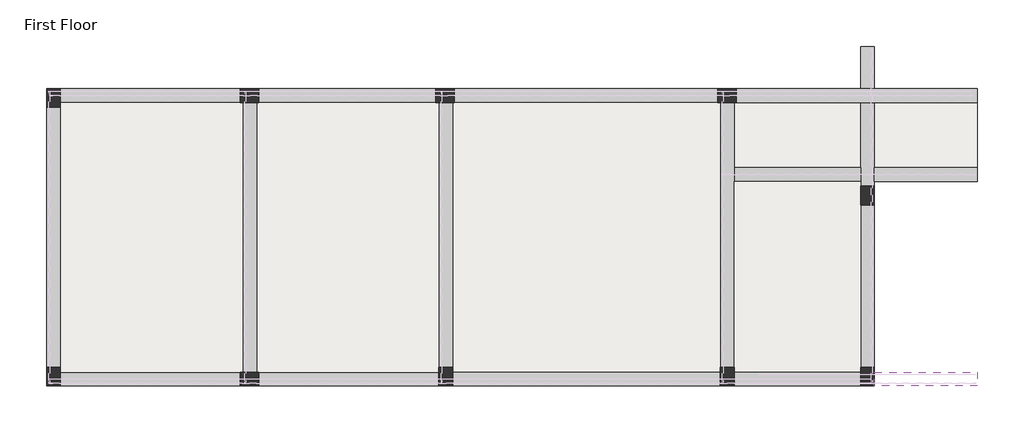
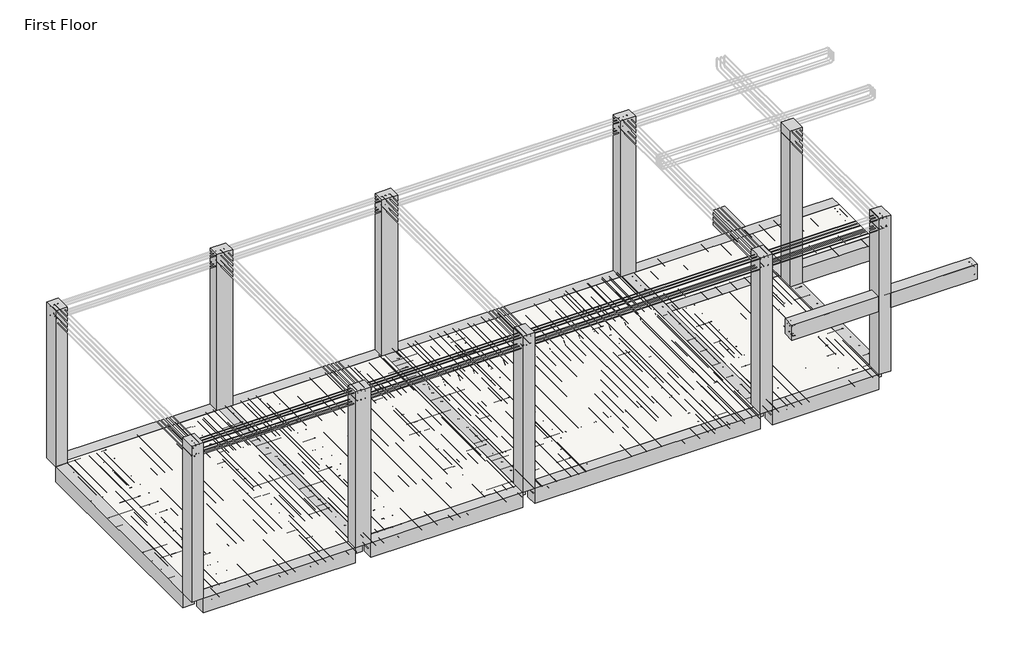
# One storey, part 1 of 4: 10 columns, 9 beams, 5 slabs.
"""IFC4 building model written with IfcOpenShell, lengths in millimetres."""

from ifc_helpers import new_model, si_unit, frame, origin, place, context, project, spatial, polyline, outline, extrude, faceted_brep, element, save

model = new_model("IFC4")

# Units and contexts
model_context = context("Model", 3, world=origin())
ifc_project = project(units=[si_unit("LENGTHUNIT", "METRE", prefix="MILLI")], contexts=[model_context])

# Site, building, storey
site = spatial("IfcSite", under=ifc_project)
building = spatial("IfcBuilding", under=site)
storey = spatial("IfcBuildingStorey", under=building, Name="First Floor", Elevation=3200.4)

# Beams
placement = place(None, origin())
element("IfcBeam", 1, ObjectType="M_Concrete-Rectangular Beam : 9\" X12\"", at=placement, inside=storey, context=model_context, shape_type="Brep", body=[
    faceted_brep([(3956.0882476, 186.4334631, 3200.4), (3956.0882476, 415.0334631, 3200.4), (1885.9882476, 415.0334631, 3200.4), (1885.9882476, 186.4334631, 3200.4), (3956.0882476, 186.4334631, 2895.6), (1885.9882476, 186.4334631, 2895.6), (3956.0882476, 415.0334631, 2895.6), (1885.9882476, 415.0334631, 2895.6), (3956.0882476, 415.0334631, 3048.0), (1885.9882476, 415.0334631, 3048.0)], [[[0, 1, 2, 3]], [[4, 0, 3, 5]], [[6, 4, 5, 7]], [[1, 8, 6, 7, 9, 2]], [[1, 0, 4, 6, 8]], [[3, 2, 9, 7, 5]]]),
    faceted_brep([(-9150.3117524, 186.4334631, 3200.4), (-9150.3117524, 415.0334631, 3200.4), (-9150.3117524, 415.0334631, 3048.0), (-9150.3117524, 415.0334631, 2895.6), (-9150.3117524, 186.4334631, 2895.6), (-6203.9117524, 415.0334631, 3200.4), (-6203.9117524, 186.4334631, 3200.4), (-6203.9117524, 186.4334631, 2895.6), (-6203.9117524, 415.0334631, 2895.6)], [[[0, 1, 2, 3, 4]], [[5, 6, 7, 8]], [[1, 0, 6, 5]], [[0, 4, 7, 6]], [[4, 3, 8, 7]], [[3, 2, 1, 5, 8]]]),
    faceted_brep([(-5899.1117524, 186.4334631, 3200.4), (-5899.1117524, 415.0334631, 3200.4), (-5899.1117524, 415.0334631, 2895.6), (-5899.1117524, 186.4334631, 2895.6), (-2952.7117524, 415.0334631, 3200.4), (-2952.7117524, 186.4334631, 3200.4), (-2952.7117524, 186.4334631, 2895.6), (-2952.7117524, 415.0334631, 2895.6), (-2952.7117524, 415.0334631, 3048.0)], [[[0, 1, 2, 3]], [[4, 5, 6, 7, 8]], [[1, 0, 5, 4]], [[0, 3, 6, 5]], [[3, 2, 7, 6]], [[2, 1, 4, 8, 7]]]),
    faceted_brep([(-2724.1117524, 186.4334631, 3200.4), (-2724.1117524, 415.0334631, 3200.4), (-2724.1117524, 415.0334631, 3048.0), (-2724.1117524, 415.0334631, 2895.6), (-2724.1117524, 186.4334631, 2895.6), (1657.3882476, 415.0334631, 3200.4), (1657.3882476, 186.4334631, 3200.4), (1657.3882476, 186.4334631, 2895.6), (1657.3882476, 415.0334631, 2895.6), (1657.3882476, 415.0334631, 3048.0)], [[[0, 1, 2, 3, 4]], [[5, 6, 7, 8, 9]], [[1, 0, 6, 5]], [[0, 4, 7, 6]], [[4, 3, 8, 7]], [[3, 2, 1, 5, 9, 8]]]),
])
element("IfcBeam", 2, ObjectType="M_Concrete-Rectangular Beam : 9\" X12\"", at=placement, inside=storey, context=model_context, shape_type="Brep", body=[
    faceted_brep([(3956.0882476, 5755.2386934, 3200.4), (4184.6882476, 5755.2386934, 3200.4), (4184.6882476, 5755.2386934, 2895.6), (3956.0882476, 5755.2386934, 2895.6), (3956.0882476, 5063.2334631, 3200.4), (4184.6882476, 5063.2334631, 3200.4), (4184.6882476, 5063.2334631, 2895.6), (3956.0882476, 5063.2334631, 2895.6)], [[[0, 1, 2, 3]], [[1, 0, 4, 5]], [[2, 1, 5, 6]], [[3, 2, 6, 7]], [[0, 3, 7, 4]], [[5, 4, 7, 6]]]),
    faceted_brep([(4184.6882476, 491.2334631, 3200.4), (3956.0882476, 491.2334631, 3200.4), (3956.0882476, 491.2334631, 2895.6), (4184.6882476, 491.2334631, 2895.6), (3956.0882476, 3158.2334631, 3200.4), (4184.6882476, 3158.2334631, 3200.4), (4184.6882476, 3158.2334631, 2895.6), (3956.0882476, 3158.2334631, 2895.6)], [[[0, 1, 2, 3]], [[4, 5, 6, 7]], [[1, 0, 5, 4]], [[0, 3, 6, 5]], [[3, 2, 7, 6]], [[2, 1, 4, 7]]]),
    faceted_brep([(4184.6882476, 3463.0334631, 3200.4), (3956.0882476, 3463.0334631, 3200.4), (3956.0882476, 3463.0334631, 2895.6), (4184.6882476, 3463.0334631, 2895.6), (3956.0882476, 4834.6334631, 3200.4), (4184.6882476, 4834.6334631, 3200.4), (4184.6882476, 4834.6334631, 3048.0), (4184.6882476, 4834.6334631, 2895.6), (3956.0882476, 4834.6334631, 2895.6), (3956.0882476, 4834.6334631, 3048.0), (4184.6882476, 3539.2334631, 3200.4), (4184.6882476, 3767.8334631, 3200.4), (3956.0882476, 3767.8334631, 3200.4), (3956.0882476, 3539.2334631, 3200.4), (4184.6882476, 3539.2334631, 2895.6), (4184.6882476, 3767.8334631, 2895.6), (3956.0882476, 3539.2334631, 2895.6), (3956.0882476, 3767.8334631, 2895.6)], [[[0, 1, 2, 3]], [[4, 5, 6, 7, 8, 9]], [[1, 0, 10, 11, 5, 4, 12, 13]], [[0, 3, 14, 15, 7, 6, 5, 11, 10]], [[3, 2, 16, 17, 8, 7, 15, 14]], [[2, 1, 13, 12, 4, 9, 8, 17, 16]]]),
])
element("IfcBeam", 3, ObjectType="M_Concrete-Rectangular Beam : 9\" X12\"", at=placement, inside=storey, context=model_context, shape_type="Brep", body=[
    faceted_brep([(5871.6882476, 4834.6334631, 3200.4), (5871.6882476, 4834.6334631, 3048.0), (5871.6882476, 4834.6334631, 2895.6), (5871.6882476, 5063.2334631, 2895.6), (5871.6882476, 5063.2334631, 3200.4), (1924.0882476, 4834.6334631, 3200.4), (1924.0882476, 5063.2334631, 3200.4), (1924.0882476, 5063.2334631, 2895.6), (1924.0882476, 4834.6334631, 2895.6), (4184.6882476, 5063.2334631, 3200.4), (3956.0882476, 5063.2334631, 3200.4), (3956.0882476, 4834.6334631, 3200.4), (4184.6882476, 4834.6334631, 3200.4), (4184.6882476, 5063.2334631, 2895.6), (3956.0882476, 5063.2334631, 2895.6), (4184.6882476, 4834.6334631, 2895.6), (3956.0882476, 4834.6334631, 2895.6)], [[[0, 1, 2, 3, 4]], [[5, 6, 7, 8]], [[0, 4, 9, 10, 6, 5, 11, 12]], [[4, 3, 13, 14, 7, 6, 10, 9]], [[3, 2, 15, 16, 8, 7, 14, 13]], [[2, 1, 0, 12, 11, 5, 8, 16, 15]]]),
    faceted_brep([(1619.2882476, 4834.6334631, 3200.4), (1619.2882476, 5063.2334631, 3200.4), (-2698.7117524, 5063.2334631, 3200.4), (-2698.7117524, 4834.6334631, 3200.4), (1619.2882476, 5063.2334631, 2895.6), (-2698.7117524, 5063.2334631, 2895.6), (1619.2882476, 4834.6334631, 2895.6), (-2698.7117524, 4834.6334631, 2895.6)], [[[0, 1, 2, 3]], [[1, 4, 5, 2]], [[4, 6, 7, 5]], [[6, 0, 3, 7]], [[1, 0, 6, 4]], [[2, 5, 7, 3]]]),
    faceted_brep([(-9150.3117524, 4834.6334631, 3200.4), (-9150.3117524, 5063.2334631, 3200.4), (-9150.3117524, 5063.2334631, 2895.6), (-9150.3117524, 4834.6334631, 2895.6), (-9150.3117524, 4834.6334631, 3048.0), (-6203.9117524, 5063.2334631, 3200.4), (-6203.9117524, 5063.2334631, 2895.6), (-6203.9117524, 4834.6334631, 3200.4), (-6203.9117524, 4834.6334631, 2895.6)], [[[0, 1, 2, 3, 4]], [[2, 1, 5, 6]], [[6, 5, 7, 8]], [[1, 0, 7, 5]], [[3, 2, 6, 8]], [[0, 4, 3, 8, 7]]]),
    faceted_brep([(-3003.5117524, 5063.2334631, 2895.6), (-3003.5117524, 5063.2334631, 3200.4), (-3003.5117524, 4834.6334631, 3200.4), (-3003.5117524, 4834.6334631, 2895.6), (-5899.1117524, 5063.2334631, 3200.4), (-5899.1117524, 5063.2334631, 2895.6), (-5899.1117524, 4834.6334631, 2895.6), (-5899.1117524, 4834.6334631, 3200.4)], [[[0, 1, 2, 3]], [[4, 5, 6, 7]], [[1, 0, 5, 4]], [[2, 1, 4, 7]], [[0, 3, 6, 5]], [[3, 2, 7, 6]]]),
])
element("IfcBeam", 4, ObjectType="M_Concrete-Rectangular Beam : 9\" X12\"", at=placement, inside=storey, context=model_context, shape_type="SweptSolid", body=[
    extrude(outline(polyline([(-9378.9117524, 4758.4334631), (-9150.3117524, 4758.4334631), (-9150.3117524, 491.2334631), (-9378.9117524, 491.2334631), (-9378.9117524, 4758.4334631)])), frame((0.0, 0.0, 2895.6), z_axis=(0.0, 0.0, 1.0), x_axis=(1.0, 0.0, 0.0)), (0.0, 0.0, 1.0), 304.8),
])
element("IfcBeam", 5, ObjectType="M_Concrete-Rectangular Beam : 9\" X12\"", at=placement, inside=storey, context=model_context, shape_type="Brep", body=[
    faceted_brep([(-6165.8117524, 415.0334631, 3200.4), (-5937.2117524, 415.0334631, 3200.4), (-5937.2117524, 4834.6334631, 3200.4), (-6165.8117524, 4834.6334631, 3200.4), (-5937.2117524, 415.0334631, 3048.0), (-5937.2117524, 415.0334631, 2895.6), (-5937.2117524, 4834.6334631, 2895.6), (-5937.2117524, 4834.6334631, 3048.0), (-6165.8117524, 415.0334631, 2895.6), (-6165.8117524, 4834.6334631, 2895.6), (-6165.8117524, 415.0334631, 3048.0), (-6165.8117524, 4834.6334631, 3048.0)], [[[0, 1, 2, 3]], [[1, 4, 5, 6, 7, 2]], [[5, 8, 9, 6]], [[8, 10, 0, 3, 11, 9]], [[1, 0, 10, 8, 5, 4]], [[3, 2, 7, 6, 9, 11]]]),
])
element("IfcBeam", 6, ObjectType="M_Concrete-Rectangular Beam : 9\" X12\"", at=placement, inside=storey, context=model_context, shape_type="Brep", body=[
    faceted_brep([(-2952.7117524, 491.2334631, 3200.4), (-2724.1117524, 491.2334631, 3200.4), (-2724.1117524, 4834.6334631, 3200.4), (-2952.7117524, 4834.6334631, 3200.4), (-2724.1117524, 491.2334631, 2895.6), (-2724.1117524, 4834.6334631, 2895.6), (-2724.1117524, 4834.6334631, 3048.0), (-2952.7117524, 491.2334631, 2895.6), (-2952.7117524, 4834.6334631, 2895.6), (-2952.7117524, 4834.6334631, 3048.0)], [[[0, 1, 2, 3]], [[1, 4, 5, 6, 2]], [[4, 7, 8, 5]], [[7, 0, 3, 9, 8]], [[1, 0, 7, 4]], [[3, 2, 6, 5, 8, 9]]]),
])
element("IfcBeam", 7, ObjectType="M_Concrete-Rectangular Beam : 9\" X12\"", at=placement, inside=storey, context=model_context, shape_type="Brep", body=[
    faceted_brep([(1657.3882476, 491.2334631, 3200.4), (1885.9882476, 491.2334631, 3200.4), (1885.9882476, 3539.2334631, 3200.4), (1885.9882476, 3767.8334631, 3200.4), (1885.9882476, 4834.6334631, 3200.4), (1657.3882476, 4834.6334631, 3200.4), (1885.9882476, 491.2334631, 2895.6), (1885.9882476, 3539.2334631, 2895.6), (1885.9882476, 3767.8334631, 2895.6), (1885.9882476, 4834.6334631, 2895.6), (1885.9882476, 4834.6334631, 3048.0), (1657.3882476, 491.2334631, 2895.6), (1657.3882476, 4834.6334631, 2895.6), (1657.3882476, 4834.6334631, 3048.0)], [[[0, 1, 2, 3, 4, 5]], [[1, 6, 7, 8, 9, 10, 4, 3, 2]], [[6, 11, 12, 9, 8, 7]], [[11, 0, 5, 13, 12]], [[1, 0, 11, 6]], [[5, 4, 10, 9, 12, 13]]]),
])
element("IfcBeam", 8, ObjectType="M_Concrete-Rectangular Beam : 9\" X12\"", at=placement, inside=storey, context=model_context, shape_type="Brep", body=[
    faceted_brep([(5871.6882476, 3539.2334631, 3200.4), (5871.6882476, 3539.2334631, 2895.6), (5871.6882476, 3767.8334631, 2895.6), (5871.6882476, 3767.8334631, 3048.0), (5871.6882476, 3767.8334631, 3200.4), (4184.6882476, 3539.2334631, 3200.4), (4184.6882476, 3767.8334631, 3200.4), (4184.6882476, 3767.8334631, 3048.0), (4184.6882476, 3767.8334631, 2895.6), (4184.6882476, 3539.2334631, 2895.6)], [[[0, 1, 2, 3, 4]], [[5, 6, 7, 8, 9]], [[0, 4, 6, 5]], [[4, 3, 2, 8, 7, 6]], [[2, 1, 9, 8]], [[1, 0, 5, 9]]]),
    faceted_brep([(1885.9882476, 3767.8334631, 3200.4), (1885.9882476, 3539.2334631, 3200.4), (3956.0882476, 3539.2334631, 3200.4), (3956.0882476, 3767.8334631, 3200.4), (1885.9882476, 3767.8334631, 2895.6), (1885.9882476, 3767.8334631, 3048.0), (3956.0882476, 3767.8334631, 3048.0), (3956.0882476, 3767.8334631, 2895.6), (1885.9882476, 3539.2334631, 2895.6), (3956.0882476, 3539.2334631, 2895.6), (1885.9882476, 3539.2334631, 3048.0), (3956.0882476, 3539.2334631, 3048.0)], [[[0, 1, 2, 3]], [[4, 5, 0, 3, 6, 7]], [[8, 4, 7, 9]], [[1, 10, 8, 9, 11, 2]], [[1, 0, 5, 4, 8, 10]], [[3, 2, 11, 9, 7, 6]]]),
])
element("IfcBeam", 9, ObjectType="M_Concrete-Rectangular Beam : 9\" X12\"", at=placement, inside=storey, context=model_context, shape_type="SweptSolid", body=[
    extrude(outline(polyline([(2271.6882476, 186.4334631), (2271.6882476, 415.0334631), (3956.0882476, 415.0334631), (3956.0882476, 186.4334631), (2271.6882476, 186.4334631)])), frame((0.0, 0.0, 4495.8), z_axis=(0.0, 0.0, 1.0), x_axis=(1.0, 0.0, 0.0)), (0.0, 0.0, 1.0), 304.8),
    extrude(outline(polyline([(5871.6882476, 415.0334631), (5871.6882476, 186.4334631), (4184.6882476, 186.4334631), (4184.6882476, 415.0334631), (5871.6882476, 415.0334631)])), frame((0.0, 0.0, 4495.8), z_axis=(0.0, 0.0, 1.0), x_axis=(1.0, 0.0, 0.0)), (0.0, 0.0, 1.0), 304.8),
])

# Columns
element("IfcColumn", 10, ObjectType="M_Concrete-Rectangular-Column : 9\" x 12\"", at=placement, inside=storey, context=model_context, shape_type="SweptSolid", body=[
    extrude(outline(polyline([(-9150.3117524, 5063.2334631), (-9150.3117524, 4758.4334631), (-9378.9117524, 4758.4334631), (-9378.9117524, 5063.2334631), (-9150.3117524, 5063.2334631)])), frame((0.0, 0.0, 3200.4), z_axis=(0.0, 0.0, 1.0), x_axis=(1.0, 0.0, 0.0)), (0.0, 0.0, 1.0), 3200.4),
])
element("IfcColumn", 11, ObjectType="M_Concrete-Rectangular-Column : 9\" x 12\"", at=placement, inside=storey, context=model_context, shape_type="SweptSolid", body=[
    extrude(outline(polyline([(-9150.3117524, 491.2334631), (-9150.3117524, 186.4334631), (-9378.9117524, 186.4334631), (-9378.9117524, 491.2334631), (-9150.3117524, 491.2334631)])), frame((0.0, 0.0, 3200.4), z_axis=(0.0, 0.0, 1.0), x_axis=(1.0, 0.0, 0.0)), (0.0, 0.0, 1.0), 3200.4),
])
element("IfcColumn", 12, ObjectType="M_Concrete-Rectangular-Column : 9\" x 12\"", at=placement, inside=storey, context=model_context, shape_type="Brep", body=[
    faceted_brep([(-6203.9117524, 415.0334631, 3200.4), (-5899.1117524, 415.0334631, 3200.4), (-5899.1117524, 186.4334631, 3200.4), (-6203.9117524, 186.4334631, 3200.4), (-6203.9117524, 415.0334631, 6400.8), (-5899.1117524, 415.0334631, 6400.8), (-5899.1117524, 415.0334631, 6096.0), (-6203.9117524, 415.0334631, 6096.0), (-5899.1117524, 186.4334631, 6400.8), (-5899.1117524, 186.4334631, 6096.0), (-6203.9117524, 186.4334631, 6400.8), (-6203.9117524, 186.4334631, 6096.0)], [[[0, 1, 2, 3]], [[4, 5, 6, 1, 0, 7]], [[5, 8, 9, 2, 1, 6]], [[8, 10, 11, 3, 2, 9]], [[10, 4, 7, 0, 3, 11]], [[4, 10, 8, 5]]]),
])
element("IfcColumn", 13, ObjectType="M_Concrete-Rectangular-Column : 9\" x 12\"", at=placement, inside=storey, context=model_context, shape_type="Brep", body=[
    faceted_brep([(-2952.7117524, 186.4334631, 3200.4), (-2952.7117524, 491.2334631, 3200.4), (-2724.1117524, 491.2334631, 3200.4), (-2724.1117524, 186.4334631, 3200.4), (-2952.7117524, 186.4334631, 6400.8), (-2952.7117524, 415.0334631, 6400.8), (-2952.7117524, 491.2334631, 6400.8), (-2952.7117524, 186.4334631, 6096.0), (-2724.1117524, 491.2334631, 6400.8), (-2724.1117524, 415.0334631, 6400.8), (-2724.1117524, 186.4334631, 6400.8), (-2724.1117524, 186.4334631, 6096.0)], [[[0, 1, 2, 3]], [[4, 5, 6, 1, 0, 7]], [[6, 8, 2, 1]], [[8, 9, 10, 11, 3, 2]], [[10, 4, 7, 0, 3, 11]], [[4, 10, 9, 8, 6, 5]]]),
])
element("IfcColumn", 14, ObjectType="M_Concrete-Rectangular-Column : 9\" x 12\"", at=placement, inside=storey, context=model_context, shape_type="Brep", body=[
    faceted_brep([(1657.3882476, 186.4334631, 3200.4), (1657.3882476, 491.2334631, 3200.4), (1885.9882476, 491.2334631, 3200.4), (1885.9882476, 186.4334631, 3200.4), (1657.3882476, 186.4334631, 6400.8), (1657.3882476, 415.0334631, 6400.8), (1657.3882476, 491.2334631, 6400.8), (1657.3882476, 186.4334631, 6096.0), (1885.9882476, 491.2334631, 6400.8), (1885.9882476, 415.0334631, 6400.8), (1885.9882476, 186.4334631, 6400.8), (1885.9882476, 186.4334631, 6096.0)], [[[0, 1, 2, 3]], [[4, 5, 6, 1, 0, 7]], [[6, 8, 2, 1]], [[8, 9, 10, 11, 3, 2]], [[10, 4, 7, 0, 3, 11]], [[4, 10, 9, 8, 6, 5]]]),
])
element("IfcColumn", 15, ObjectType="M_Concrete-Rectangular-Column : 9\" x 12\"", at=placement, inside=storey, context=model_context, shape_type="Brep", body=[
    faceted_brep([(3956.0882476, 186.4334631, 3200.4), (3956.0882476, 491.2334631, 3200.4), (4184.6882476, 491.2334631, 3200.4), (4184.6882476, 186.4334631, 3200.4), (3956.0882476, 186.4334631, 6400.8), (3956.0882476, 491.2334631, 6400.8), (3956.0882476, 186.4334631, 4495.8), (3956.0882476, 186.4334631, 4800.6), (4184.6882476, 491.2334631, 6400.8), (4184.6882476, 186.4334631, 6400.8), (4184.6882476, 186.4334631, 4800.6), (4184.6882476, 186.4334631, 4495.8)], [[[0, 1, 2, 3]], [[4, 5, 1, 0, 6, 7]], [[5, 8, 2, 1]], [[8, 9, 10, 11, 3, 2]], [[9, 4, 7, 6, 0, 3, 11, 10]], [[4, 9, 8, 5]]]),
])
element("IfcColumn", 16, ObjectType="M_Concrete-Rectangular-Column : 9\" x 12\"", at=placement, inside=storey, context=model_context, shape_type="Brep", body=[
    faceted_brep([(3956.0882476, 3158.2334631, 3200.4), (3956.0882476, 3463.0334631, 3200.4), (4184.6882476, 3463.0334631, 3200.4), (4184.6882476, 3158.2334631, 3200.4), (3956.0882476, 3158.2334631, 6400.8), (3956.0882476, 3463.0334631, 6400.8), (3956.0882476, 3463.0334631, 6096.0), (3956.0882476, 3158.2334631, 6096.0), (4184.6882476, 3463.0334631, 6400.8), (4184.6882476, 3463.0334631, 6096.0), (4184.6882476, 3158.2334631, 6400.8), (4184.6882476, 3158.2334631, 6096.0)], [[[0, 1, 2, 3]], [[4, 5, 6, 1, 0, 7]], [[5, 8, 9, 2, 1, 6]], [[8, 10, 11, 3, 2, 9]], [[10, 4, 7, 0, 3, 11]], [[4, 10, 8, 5]]]),
])
element("IfcColumn", 17, ObjectType="M_Concrete-Rectangular-Column : 9\" x 12\"", at=placement, inside=storey, context=model_context, shape_type="Brep", body=[
    faceted_brep([(1924.0882476, 4834.6334631, 3200.4), (1619.2882476, 4834.6334631, 3200.4), (1619.2882476, 5063.2334631, 3200.4), (1924.0882476, 5063.2334631, 3200.4), (1924.0882476, 4834.6334631, 6400.8), (1619.2882476, 4834.6334631, 6400.8), (1619.2882476, 4834.6334631, 6096.0), (1924.0882476, 4834.6334631, 6096.0), (1619.2882476, 5063.2334631, 6400.8), (1619.2882476, 5063.2334631, 6096.0), (1924.0882476, 5063.2334631, 6400.8), (1924.0882476, 5063.2334631, 6096.0)], [[[0, 1, 2, 3]], [[4, 5, 6, 1, 0, 7]], [[5, 8, 9, 2, 1, 6]], [[8, 10, 11, 3, 2, 9]], [[10, 4, 7, 0, 3, 11]], [[4, 10, 8, 5]]]),
])
element("IfcColumn", 18, ObjectType="M_Concrete-Rectangular-Column : 9\" x 12\"", at=placement, inside=storey, context=model_context, shape_type="Brep", body=[
    faceted_brep([(-2698.7117524, 4834.6334631, 3200.4), (-3003.5117524, 4834.6334631, 3200.4), (-3003.5117524, 5063.2334631, 3200.4), (-2698.7117524, 5063.2334631, 3200.4), (-2698.7117524, 4834.6334631, 6400.8), (-3003.5117524, 4834.6334631, 6400.8), (-3003.5117524, 4834.6334631, 6096.0), (-2698.7117524, 4834.6334631, 6096.0), (-3003.5117524, 5063.2334631, 6400.8), (-3003.5117524, 5063.2334631, 6096.0), (-2698.7117524, 5063.2334631, 6400.8), (-2698.7117524, 5063.2334631, 6096.0)], [[[0, 1, 2, 3]], [[4, 5, 6, 1, 0, 7]], [[5, 8, 9, 2, 1, 6]], [[8, 10, 11, 3, 2, 9]], [[10, 4, 7, 0, 3, 11]], [[4, 10, 8, 5]]]),
])
element("IfcColumn", 19, ObjectType="M_Concrete-Rectangular-Column : 9\" x 12\"", at=placement, inside=storey, context=model_context, shape_type="Brep", body=[
    faceted_brep([(-5899.1117524, 4834.6334631, 3200.4), (-6203.9117524, 4834.6334631, 3200.4), (-6203.9117524, 5063.2334631, 3200.4), (-5899.1117524, 5063.2334631, 3200.4), (-5899.1117524, 4834.6334631, 6400.8), (-6203.9117524, 4834.6334631, 6400.8), (-6203.9117524, 4834.6334631, 6096.0), (-5899.1117524, 4834.6334631, 6096.0), (-6203.9117524, 5063.2334631, 6400.8), (-6203.9117524, 5063.2334631, 6096.0), (-5899.1117524, 5063.2334631, 6400.8), (-5899.1117524, 5063.2334631, 6096.0)], [[[0, 1, 2, 3]], [[4, 5, 6, 1, 0, 7]], [[5, 8, 9, 2, 1, 6]], [[8, 10, 11, 3, 2, 9]], [[10, 4, 7, 0, 3, 11]], [[4, 10, 8, 5]]]),
])

# Slabs
element("IfcSlab", 20, ObjectType="FLOOR SLAB 6\"", at=placement, inside=storey, context=model_context, shape_type="Brep", body=[
    faceted_brep([(-6165.8117524, 4834.6334631, 3048.0), (-6165.8117524, 415.0334631, 3048.0), (-9150.3117524, 415.0334631, 3048.0), (-9150.3117524, 4834.6334631, 3048.0), (-6165.8117524, 4834.6334631, 3200.4), (-6203.9117524, 4834.6334631, 3200.4), (-9150.3117524, 4834.6334631, 3200.4), (-9150.3117524, 4758.4334631, 3200.4), (-9150.3117524, 491.2334631, 3200.4), (-9150.3117524, 415.0334631, 3200.4), (-6203.9117524, 415.0334631, 3200.4), (-6165.8117524, 415.0334631, 3200.4)], [[[0, 1, 2, 3]], [[4, 5, 6, 7, 8, 9, 10, 11]], [[1, 0, 4, 11]], [[2, 1, 11, 10, 9]], [[3, 2, 9, 8, 7, 6]], [[0, 3, 6, 5, 4]]]),
])
element("IfcSlab", 21, ObjectType="FLOOR SLAB 6\"", at=placement, inside=storey, context=model_context, shape_type="Brep", body=[
    faceted_brep([(-2952.7117524, 4834.6334631, 3048.0), (-2952.7117524, 415.0334631, 3048.0), (-5937.2117524, 415.0334631, 3048.0), (-5937.2117524, 4834.6334631, 3048.0), (-2952.7117524, 4834.6334631, 3200.4), (-3003.5117524, 4834.6334631, 3200.4), (-5899.1117524, 4834.6334631, 3200.4), (-5937.2117524, 4834.6334631, 3200.4), (-5937.2117524, 415.0334631, 3200.4), (-5899.1117524, 415.0334631, 3200.4), (-2952.7117524, 415.0334631, 3200.4), (-2952.7117524, 491.2334631, 3200.4)], [[[0, 1, 2, 3]], [[4, 5, 6, 7, 8, 9, 10, 11]], [[1, 0, 4, 11, 10]], [[2, 1, 10, 9, 8]], [[3, 2, 8, 7]], [[0, 3, 7, 6, 5, 4]]]),
])
element("IfcSlab", 22, ObjectType="FLOOR SLAB 6\"", at=placement, inside=storey, context=model_context, shape_type="Brep", body=[
    faceted_brep([(1657.3882476, 4834.6334631, 3048.0), (1657.3882476, 415.0334631, 3048.0), (-2724.1117524, 415.0334631, 3048.0), (-2724.1117524, 4834.6334631, 3048.0), (1657.3882476, 4834.6334631, 3200.4), (1619.2882476, 4834.6334631, 3200.4), (-2698.7117524, 4834.6334631, 3200.4), (-2724.1117524, 4834.6334631, 3200.4), (-2724.1117524, 491.2334631, 3200.4), (-2724.1117524, 415.0334631, 3200.4), (1657.3882476, 415.0334631, 3200.4), (1657.3882476, 491.2334631, 3200.4)], [[[0, 1, 2, 3]], [[4, 5, 6, 7, 8, 9, 10, 11]], [[1, 0, 4, 11, 10]], [[2, 1, 10, 9]], [[3, 2, 9, 8, 7]], [[0, 3, 7, 6, 5, 4]]]),
])
element("IfcSlab", 23, ObjectType="FLOOR SLAB 6\"", at=placement, inside=storey, context=model_context, shape_type="Brep", body=[
    faceted_brep([(3956.0882476, 415.0334631, 3048.0), (1885.9882476, 415.0334631, 3048.0), (1885.9882476, 3539.2334631, 3048.0), (3956.0882476, 3539.2334631, 3048.0), (3956.0882476, 415.0334631, 3200.4), (3956.0882476, 491.2334631, 3200.4), (3956.0882476, 3158.2334631, 3200.4), (3956.0882476, 3463.0334631, 3200.4), (3956.0882476, 3539.2334631, 3200.4), (1885.9882476, 3539.2334631, 3200.4), (1885.9882476, 491.2334631, 3200.4), (1885.9882476, 415.0334631, 3200.4)], [[[0, 1, 2, 3]], [[4, 5, 6, 7, 8, 9, 10, 11]], [[1, 0, 4, 11]], [[2, 1, 11, 10, 9]], [[3, 2, 9, 8]], [[0, 3, 8, 7, 6, 5, 4]]]),
])
element("IfcSlab", 24, ObjectType="FLOOR SLAB 6\"", at=placement, inside=storey, context=model_context, shape_type="Brep", body=[
    faceted_brep([(3956.0882476, 3767.8334631, 3048.0), (1885.9882476, 3767.8334631, 3048.0), (1885.9882476, 4834.6334631, 3048.0), (3956.0882476, 4834.6334631, 3048.0), (3956.0882476, 3767.8334631, 3200.4), (3956.0882476, 4834.6334631, 3200.4), (1924.0882476, 4834.6334631, 3200.4), (1885.9882476, 4834.6334631, 3200.4), (1885.9882476, 3767.8334631, 3200.4)], [[[0, 1, 2, 3]], [[4, 5, 6, 7, 8]], [[1, 0, 4, 8]], [[2, 1, 8, 7]], [[3, 2, 7, 6, 5]], [[0, 3, 5, 4]]]),
    faceted_brep([(5871.6882476, 4834.6334631, 3048.0), (5871.6882476, 3767.8334631, 3048.0), (4184.6882476, 3767.8334631, 3048.0), (4184.6882476, 4834.6334631, 3048.0), (5871.6882476, 4834.6334631, 3200.4), (4184.6882476, 4834.6334631, 3200.4), (4184.6882476, 3767.8334631, 3200.4), (5871.6882476, 3767.8334631, 3200.4)], [[[0, 1, 2, 3]], [[4, 5, 6, 7]], [[1, 0, 4, 7]], [[2, 1, 7, 6]], [[3, 2, 6, 5]], [[0, 3, 5, 4]]]),
])

save(model, "model.ifc")

# Revit data of these elements
# Type "M_Concrete-Rectangular Beam : 9\" X12\""
#   Length [instance default] = 5' - 0"
#   b = 0' - 9"
#   h = 1' - 0"
#   Structural Material [instance default] = Concrete, Cast-in-Place gray
#   Assembly Code = ""
# Type "M_Concrete-Rectangular-Column : 9\" x 12\""
#   b = 0' - 9"
#   h = 1' - 0"
#   Structural Material [instance default] = Concrete, Cast-in-Place gray
# Type "FLOOR SLAB 6\""
#   Layers, outside or top first: 0' - 6" "Concrete, Cast-in-Place gray" (function 1)
# Elements 1, 2, 3, 4, 5, 6, 7, 8, 9 (IfcBeam, "M_Concrete-Rectangular Beam : 9\" X12\"")
#   Structural Material = Concrete, Cast-in-Place gray
#   Phase Created = New Construction
#   Materials on its faces: "Concrete, Cast-in-Place gray"
# Elements 10, 11, 12, 13, 14, 15, 16, 17, 18, 19 (IfcColumn, "M_Concrete-Rectangular-Column : 9\" x 12\"")
#   Structural Material = Concrete, Cast-in-Place gray
#   Phase Created = New Construction
#   Materials on its faces: "Concrete, Cast-in-Place gray"
# Elements 20, 21, 22, 23, 24 (IfcSlab, "FLOOR SLAB 6\"")
#   Height Offset From Level = 0' - 0"
#   built-in parameter 1001954 = 1
#   Phase Created = New Construction
#   Materials on its faces: "Concrete, Cast-in-Place gray"
# Materials
#   "Concrete, Cast-in-Place gray": class "Concrete", colour RGB 192 192 192, transparency 0, Description = "Cast-in-place concrete", Cost = 0
